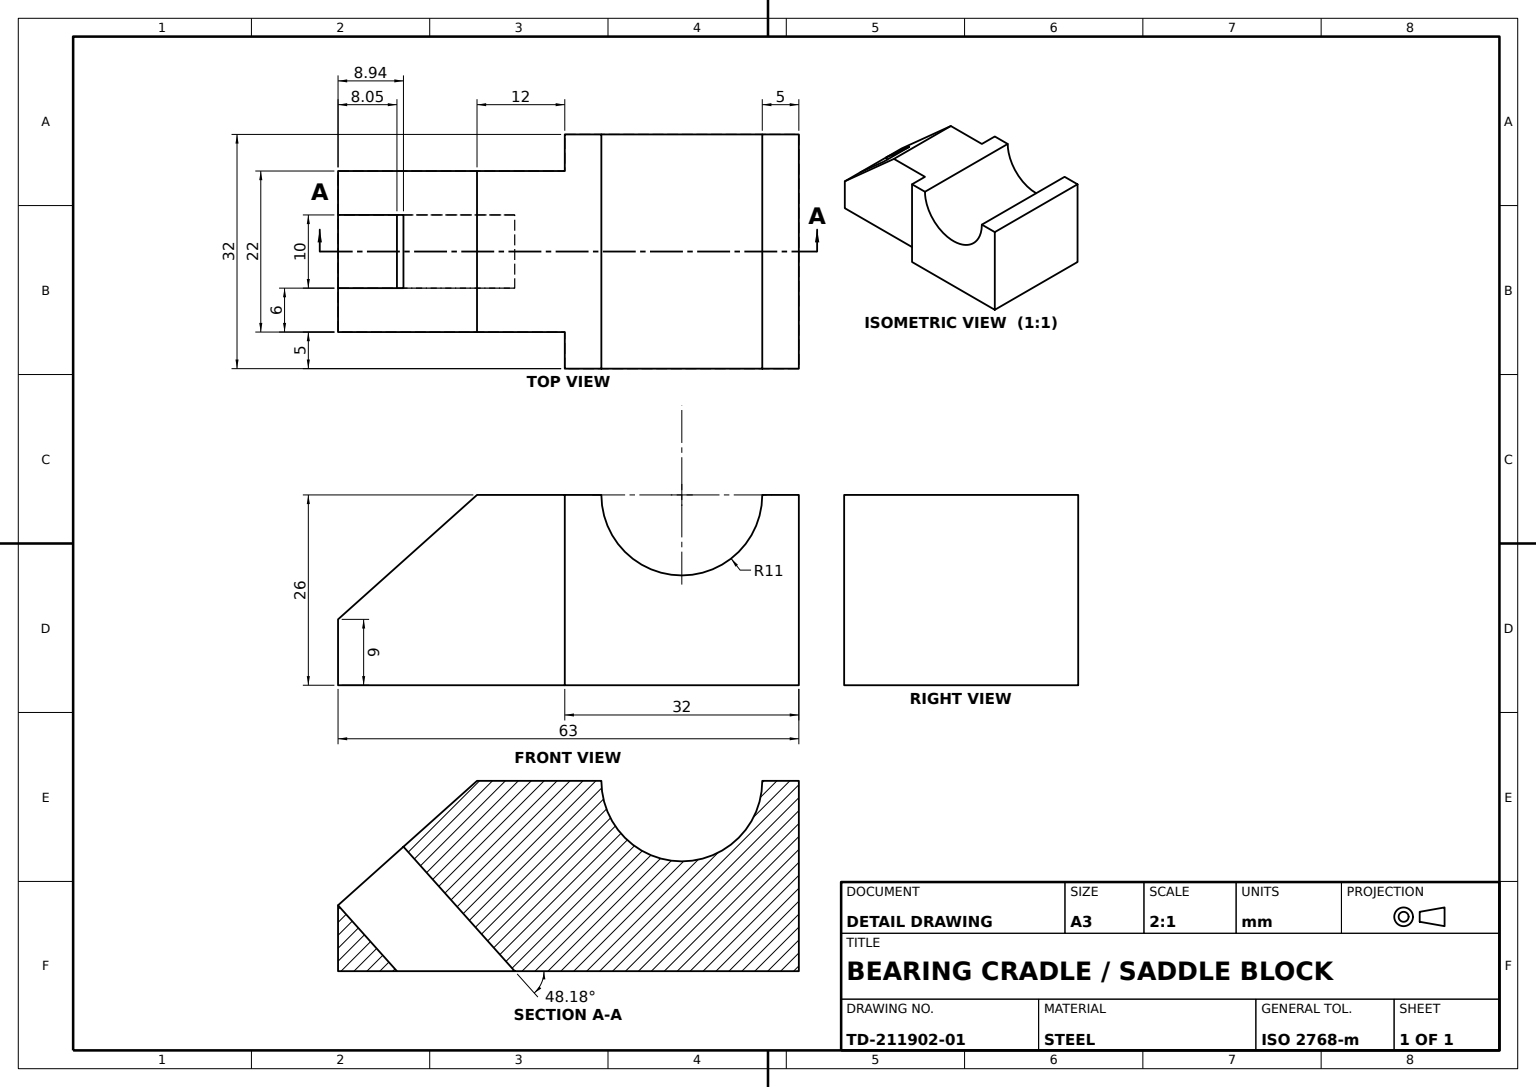
from build123d import *

# Parameters (mm, degrees)
CRADLE_BLOCK_DEPTH      = 16
TAPERED_EXTENSION_DEPTH = 11
RELIEF_SLOT_PROFILE_W   = 12
RELIEF_SLOT_PROFILE_H   = 10
RELIEF_SLOT_DEPTH       = 52.378729511


with BuildPart() as part:
    # Cradle Block Profile → Cradle Block (new, symmetric)
    with BuildSketch(Plane.XY):
        with BuildLine():
            Line((11, 13), (16, 13))
            Line((16, 13), (16, -13))
            Line((16, -13), (-16, -13))
            Line((-16, -13), (-16, 13))
            Line((-16, 13), (-11, 13))
            ThreePointArc((-11, 13), (0, 2), (11, 13))
        make_face()
    extrude(amount=CRADLE_BLOCK_DEPTH, both=True)

    # Tapered Extension Profile → Tapered Extension (add, symmetric)
    with BuildSketch(Plane.XY):
        Polygon((-16, 13), (-28, 13), (-47, -4), (-47, -13), (-16, -13), align=None)
    extrude(amount=TAPERED_EXTENSION_DEPTH, both=True)

    # Relief Slot Profile → Relief Slot (cut, through all)
    with BuildSketch(Plane(origin=(-18.909230769, 21.133846154, 0), x_dir=(0.745241313525099, 0.6667948594698261, 0), z_dir=(-0.6667948594698261, 0.745241313525099, 0))):
        with Locations((-31.693521174, 0)):
            Rectangle(RELIEF_SLOT_PROFILE_W, RELIEF_SLOT_PROFILE_H)
    extrude(amount=-RELIEF_SLOT_DEPTH, mode=Mode.SUBTRACT)


solid = part.part
